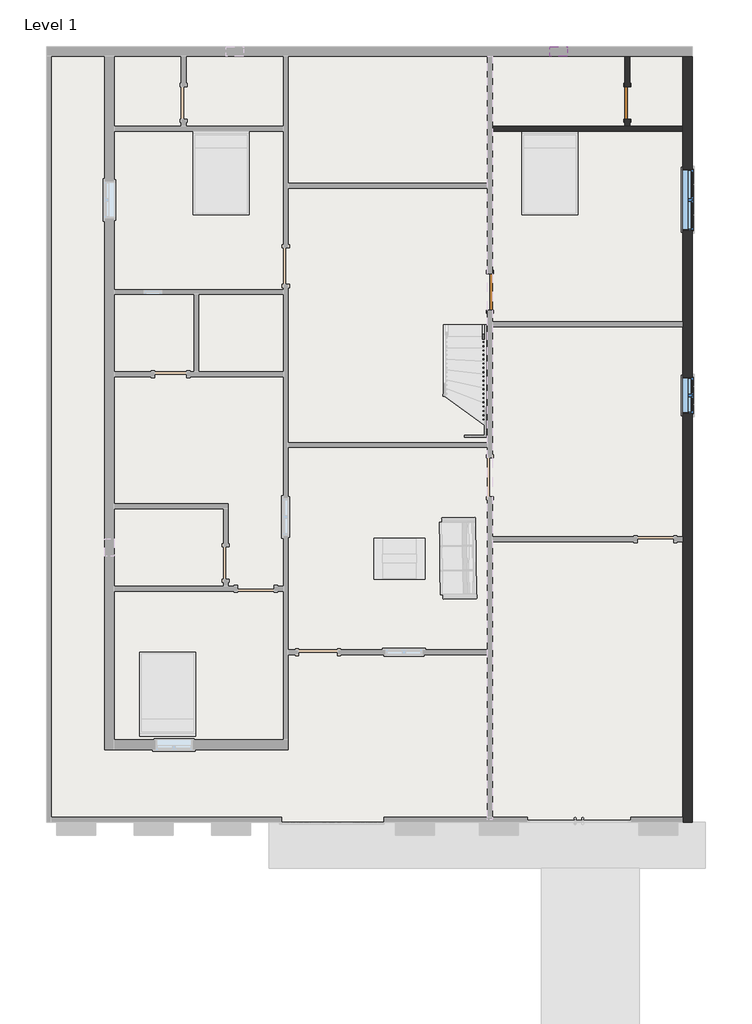
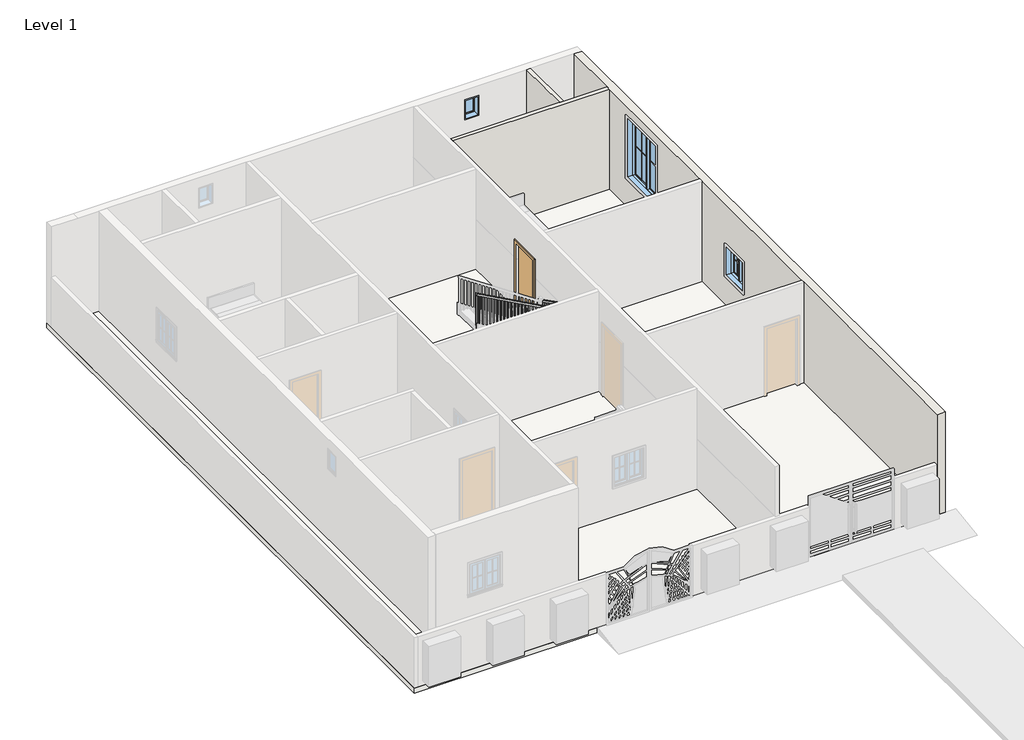
# One storey, part 2 of 3: 3 walls, 3 windows, 2 doors, 1 railing, 1 slab.
"""IFC4 building model written with IfcOpenShell, lengths in millimetres."""

from ifc_helpers import new_model, si_unit, frame, origin, place, context, project, spatial, polyline, outline, extrude, faceted_brep, transform, mapped, element, save
from components import door_f2b275c1, door_c29894e6, window_aa618e30, window_339605e1, window_9ac97e1a

model = new_model("IFC4")

# Units and contexts
model_context = context("Model", 3, world=origin())
ifc_project = project(units=[si_unit("LENGTHUNIT", "METRE", prefix="MILLI")], contexts=[model_context])

# Site, building, storey
site = spatial("IfcSite", under=ifc_project)
building = spatial("IfcBuilding", under=site)
storey = spatial("IfcBuildingStorey", under=building, Name="Level 1", Elevation=0.0)

# Doors
placement = place(None, origin())
door_shape = door_f2b275c1(model_context)
element("IfcDoor", 1, ObjectType="Single-Flush : 30\" x 80\"", at=placement, inside=storey, context=model_context, shape_type="MappedRepresentation", body=[
    mapped(door_shape, transform((4827.3366507, 9100.7522623, 0.0), x_axis=(0.0, -1.0, 0.0), y_axis=(1.0, 0.0, 0.0), z_axis=(0.0, 0.0, 1.0))),
])
door_2_shape = door_c29894e6(model_context)
element("IfcDoor", 2, ObjectType="Single-Flush : 34\" x 80\"", at=placement, inside=storey, context=model_context, shape_type="MappedRepresentation", body=[
    mapped(door_2_shape, transform((1583.2084916, 4643.0522623, 0.0), x_axis=(0.0, -1.0, 0.0), y_axis=(1.0, 0.0, 0.0), z_axis=(0.0, 0.0, 1.0))),
])

# Railing
element("IfcRailing", 3, ObjectType="Handrail - Rectangular", at=placement, inside=storey, context=model_context, shape_type="SolidModel", body=[
    faceted_brep([(1456.2084916, 3870.4222402, 1083.7333333), (1456.2084916, 3870.4222402, 1026.7391458), (1405.4084916, 3870.4222402, 1026.7391458), (1405.4084916, 3870.4222402, 1083.7333333), (1456.2084916, 1506.6647172, 2286.078212), (1456.2084916, 1494.487215, 2235.278212), (1405.4084916, 1494.487215, 2235.278212), (1405.4084916, 1506.6647172, 2286.078212), (1456.2084916, 1268.9652728, 2286.078212), (1456.2084916, 1268.9652728, 2235.278212), (1405.4084916, 1319.7652728, 2235.278212), (1405.4084916, 1319.7652728, 2286.078212), (1234.4478889, 1268.9652728, 2286.078212), (1221.4006723, 1268.9652728, 2235.278212), (1221.4006723, 1319.7652728, 2235.278212), (1234.4478889, 1319.7652728, 2286.078212), (-1813.7050583, 1268.9652728, 3962.4), (-1813.7050583, 1319.7652728, 3962.4), (-1813.7050583, 1319.7652728, 3904.4247257), (-1813.7050583, 1268.9652728, 3904.4247257)], [[[0, 1, 2, 3]], [[1, 0, 4, 5]], [[2, 1, 5, 6]], [[3, 2, 6, 7]], [[0, 3, 7, 4]], [[5, 4, 8, 9]], [[6, 5, 9, 10]], [[7, 6, 10, 11]], [[4, 7, 11, 8]], [[9, 8, 12, 13]], [[10, 9, 13, 14]], [[11, 10, 14, 15]], [[8, 11, 15, 12]], [[16, 17, 18, 19]], [[13, 12, 16, 19]], [[14, 13, 19, 18]], [[15, 14, 18, 17]], [[12, 15, 17, 16]]]),
    extrude(outline(polyline([(3857.4655707, -1728.3165084), (2878.6666667, -1728.3165084), (2878.6666667, -1709.2665084), (3846.9890853, -1709.2665084), (3857.4655707, -1728.3165084)])), frame((0.0, 1284.8402728, 0.0), z_axis=(0.0, 1.0, 0.0), x_axis=(0.0, 0.0, 1.0)), (0.0, 0.0, 1.0), 19.05),
    extrude(outline(polyline([(3801.5909816, -1626.7165084), (2878.6666667, -1626.7165084), (2878.6666667, -1607.6665084), (3791.1144961, -1607.6665084), (3801.5909816, -1626.7165084)])), frame((0.0, 1284.8402728, 0.0), z_axis=(0.0, 1.0, 0.0), x_axis=(0.0, 0.0, 1.0)), (0.0, 0.0, 1.0), 19.05),
    extrude(outline(polyline([(3745.7163924, -1525.1165084), (2709.3333333, -1525.1165084), (2709.3333333, -1506.0665084), (3735.2399069, -1506.0665084), (3745.7163924, -1525.1165084)])), frame((0.0, 1284.8402728, 0.0), z_axis=(0.0, 1.0, 0.0), x_axis=(0.0, 0.0, 1.0)), (0.0, 0.0, 1.0), 19.05),
    extrude(outline(polyline([(3689.8418032, -1423.5165084), (2709.3333333, -1423.5165084), (2709.3333333, -1404.4665084), (3679.3653177, -1404.4665084), (3689.8418032, -1423.5165084)])), frame((0.0, 1284.8402728, 0.0), z_axis=(0.0, 1.0, 0.0), x_axis=(0.0, 0.0, 1.0)), (0.0, 0.0, 1.0), 19.05),
    extrude(outline(polyline([(3633.967214, -1321.9165084), (2709.3333333, -1321.9165084), (2709.3333333, -1302.8665084), (3623.4907286, -1302.8665084), (3633.967214, -1321.9165084)])), frame((0.0, 1284.8402728, 0.0), z_axis=(0.0, 1.0, 0.0), x_axis=(0.0, 0.0, 1.0)), (0.0, 0.0, 1.0), 19.05),
    extrude(outline(polyline([(3578.0926249, -1220.3165084), (2540.0, -1220.3165084), (2540.0, -1201.2665084), (3567.6161394, -1201.2665084), (3578.0926249, -1220.3165084)])), frame((0.0, 1284.8402728, 0.0), z_axis=(0.0, 1.0, 0.0), x_axis=(0.0, 0.0, 1.0)), (0.0, 0.0, 1.0), 19.05),
    extrude(outline(polyline([(3522.2180357, -1118.7165084), (2540.0, -1118.7165084), (2540.0, -1099.6665084), (3511.7415502, -1099.6665084), (3522.2180357, -1118.7165084)])), frame((0.0, 1284.8402728, 0.0), z_axis=(0.0, 1.0, 0.0), x_axis=(0.0, 0.0, 1.0)), (0.0, 0.0, 1.0), 19.05),
    extrude(outline(polyline([(3466.3434465, -1017.1165084), (2540.0, -1017.1165084), (2540.0, -998.0665084), (3455.866961, -998.0665084), (3466.3434465, -1017.1165084)])), frame((0.0, 1284.8402728, 0.0), z_axis=(0.0, 1.0, 0.0), x_axis=(0.0, 0.0, 1.0)), (0.0, 0.0, 1.0), 19.05),
    extrude(outline(polyline([(3410.4688573, -915.5165084), (2370.6666667, -915.5165084), (2370.6666667, -896.4665084), (3399.9923719, -896.4665084), (3410.4688573, -915.5165084)])), frame((0.0, 1284.8402728, 0.0), z_axis=(0.0, 1.0, 0.0), x_axis=(0.0, 0.0, 1.0)), (0.0, 0.0, 1.0), 19.05),
    extrude(outline(polyline([(3354.5942682, -813.9165084), (2370.6666667, -813.9165084), (2370.6666667, -794.8665084), (3344.1177827, -794.8665084), (3354.5942682, -813.9165084)])), frame((0.0, 1284.8402728, 0.0), z_axis=(0.0, 1.0, 0.0), x_axis=(0.0, 0.0, 1.0)), (0.0, 0.0, 1.0), 19.05),
    extrude(outline(polyline([(3298.719679, -712.3165084), (2370.6666667, -712.3165084), (2370.6666667, -693.2665084), (3288.2431935, -693.2665084), (3298.719679, -712.3165084)])), frame((0.0, 1284.8402728, 0.0), z_axis=(0.0, 1.0, 0.0), x_axis=(0.0, 0.0, 1.0)), (0.0, 0.0, 1.0), 19.05),
    extrude(outline(polyline([(3242.8450898, -610.7165084), (2201.3333333, -610.7165084), (2201.3333333, -591.6665084), (3232.3686044, -591.6665084), (3242.8450898, -610.7165084)])), frame((0.0, 1284.8402728, 0.0), z_axis=(0.0, 1.0, 0.0), x_axis=(0.0, 0.0, 1.0)), (0.0, 0.0, 1.0), 19.05),
    extrude(outline(polyline([(3186.9705007, -509.1165084), (2201.3333333, -509.1165084), (2201.3333333, -490.0665084), (3176.4940152, -490.0665084), (3186.9705007, -509.1165084)])), frame((0.0, 1284.8402728, 0.0), z_axis=(0.0, 1.0, 0.0), x_axis=(0.0, 0.0, 1.0)), (0.0, 0.0, 1.0), 19.05),
    extrude(outline(polyline([(3131.0959115, -407.5165084), (2201.3333333, -407.5165084), (2201.3333333, -388.4665084), (3120.619426, -388.4665084), (3131.0959115, -407.5165084)])), frame((0.0, 1284.8402728, 0.0), z_axis=(0.0, 1.0, 0.0), x_axis=(0.0, 0.0, 1.0)), (0.0, 0.0, 1.0), 19.05),
    extrude(outline(polyline([(3075.2213223, -305.9165084), (2032.0, -305.9165084), (2032.0, -286.8665084), (3064.7448368, -286.8665084), (3075.2213223, -305.9165084)])), frame((0.0, 1284.8402728, 0.0), z_axis=(0.0, 1.0, 0.0), x_axis=(0.0, 0.0, 1.0)), (0.0, 0.0, 1.0), 19.05),
    extrude(outline(polyline([(3019.3467331, -204.3165084), (2032.0, -204.3165084), (2032.0, -185.2665084), (3008.8702477, -185.2665084), (3019.3467331, -204.3165084)])), frame((0.0, 1284.8402728, 0.0), z_axis=(0.0, 1.0, 0.0), x_axis=(0.0, 0.0, 1.0)), (0.0, 0.0, 1.0), 19.05),
    extrude(outline(polyline([(2963.472144, -102.7165084), (2032.0, -102.7165084), (2032.0, -83.6665084), (2952.9956585, -83.6665084), (2963.472144, -102.7165084)])), frame((0.0, 1284.8402728, 0.0), z_axis=(0.0, 1.0, 0.0), x_axis=(0.0, 0.0, 1.0)), (0.0, 0.0, 1.0), 19.05),
    extrude(outline(polyline([(2907.5975548, -1.1165084), (1862.6666667, -1.1165084), (1862.6666667, 17.9334916), (2897.1210693, 17.9334916), (2907.5975548, -1.1165084)])), frame((0.0, 1284.8402728, 0.0), z_axis=(0.0, 1.0, 0.0), x_axis=(0.0, 0.0, 1.0)), (0.0, 0.0, 1.0), 19.05),
    extrude(outline(polyline([(2851.7229656, 100.4834916), (1862.6666667, 100.4834916), (1862.6666667, 119.5334916), (2841.2464801, 119.5334916), (2851.7229656, 100.4834916)])), frame((0.0, 1284.8402728, 0.0), z_axis=(0.0, 1.0, 0.0), x_axis=(0.0, 0.0, 1.0)), (0.0, 0.0, 1.0), 19.05),
    extrude(outline(polyline([(2795.8483764, 202.0834916), (1862.6666667, 202.0834916), (1862.6666667, 221.1334916), (2785.371891, 221.1334916), (2795.8483764, 202.0834916)])), frame((0.0, 1284.8402728, 0.0), z_axis=(0.0, 1.0, 0.0), x_axis=(0.0, 0.0, 1.0)), (0.0, 0.0, 1.0), 19.05),
    extrude(outline(polyline([(2739.9737873, 303.6834916), (1693.3333333, 303.6834916), (1693.3333333, 322.7334916), (2729.4973018, 322.7334916), (2739.9737873, 303.6834916)])), frame((0.0, 1284.8402728, 0.0), z_axis=(0.0, 1.0, 0.0), x_axis=(0.0, 0.0, 1.0)), (0.0, 0.0, 1.0), 19.05),
    extrude(outline(polyline([(2684.0991981, 405.2834916), (1693.3333333, 405.2834916), (1693.3333333, 424.3334916), (2673.6227126, 424.3334916), (2684.0991981, 405.2834916)])), frame((0.0, 1284.8402728, 0.0), z_axis=(0.0, 1.0, 0.0), x_axis=(0.0, 0.0, 1.0)), (0.0, 0.0, 1.0), 19.05),
    extrude(outline(polyline([(2628.2246089, 506.8834916), (1693.3333333, 506.8834916), (1693.3333333, 525.9334916), (2617.7481235, 525.9334916), (2628.2246089, 506.8834916)])), frame((0.0, 1284.8402728, 0.0), z_axis=(0.0, 1.0, 0.0), x_axis=(0.0, 0.0, 1.0)), (0.0, 0.0, 1.0), 19.05),
    extrude(outline(polyline([(2572.3500198, 608.4834916), (1524.0, 608.4834916), (1524.0, 627.5334916), (2561.8735343, 627.5334916), (2572.3500198, 608.4834916)])), frame((0.0, 1284.8402728, 0.0), z_axis=(0.0, 1.0, 0.0), x_axis=(0.0, 0.0, 1.0)), (0.0, 0.0, 1.0), 19.05),
    extrude(outline(polyline([(2516.4754306, 710.0834916), (1524.0, 710.0834916), (1524.0, 729.1334916), (2505.9989451, 729.1334916), (2516.4754306, 710.0834916)])), frame((0.0, 1284.8402728, 0.0), z_axis=(0.0, 1.0, 0.0), x_axis=(0.0, 0.0, 1.0)), (0.0, 0.0, 1.0), 19.05),
    extrude(outline(polyline([(2460.6008414, 811.6834916), (1524.0, 811.6834916), (1524.0, 830.7334916), (2450.1243559, 830.7334916), (2460.6008414, 811.6834916)])), frame((0.0, 1284.8402728, 0.0), z_axis=(0.0, 1.0, 0.0), x_axis=(0.0, 0.0, 1.0)), (0.0, 0.0, 1.0), 19.05),
    extrude(outline(polyline([(2404.7262522, 913.2834916), (1524.0, 913.2834916), (1524.0, 932.3334916), (2394.2497668, 932.3334916), (2404.7262522, 913.2834916)])), frame((0.0, 1284.8402728, 0.0), z_axis=(0.0, 1.0, 0.0), x_axis=(0.0, 0.0, 1.0)), (0.0, 0.0, 1.0), 19.05),
    extrude(outline(polyline([(2348.8516631, 1014.8834916), (1354.6666667, 1014.8834916), (1354.6666667, 1033.9334916), (2338.3751776, 1033.9334916), (2348.8516631, 1014.8834916)])), frame((0.0, 1284.8402728, 0.0), z_axis=(0.0, 1.0, 0.0), x_axis=(0.0, 0.0, 1.0)), (0.0, 0.0, 1.0), 19.05),
    extrude(outline(polyline([(2292.9770739, 1116.4834916), (1354.6666667, 1116.4834916), (1354.6666667, 1135.5334916), (2282.5005884, 1135.5334916), (2292.9770739, 1116.4834916)])), frame((0.0, 1284.8402728, 0.0), z_axis=(0.0, 1.0, 0.0), x_axis=(0.0, 0.0, 1.0)), (0.0, 0.0, 1.0), 19.05),
    extrude(outline(polyline([(2237.1024847, 1218.0834916), (1354.6666667, 1218.0834916), (1354.6666667, 1237.1334916), (2226.6259992, 1237.1334916), (2237.1024847, 1218.0834916)])), frame((0.0, 1284.8402728, 0.0), z_axis=(0.0, 1.0, 0.0), x_axis=(0.0, 0.0, 1.0)), (0.0, 0.0, 1.0), 19.05),
    extrude(outline(polyline([(1338.7334916, 1284.8402728), (1319.6834916, 1284.8402728), (1319.6834916, 1303.8902728), (1338.7334916, 1303.8902728), (1338.7334916, 1284.8402728)])), frame((0.0, 0.0, 1354.6666667), z_axis=(0.0, 0.0, 1.0), x_axis=(1.0, 0.0, 0.0)), (0.0, 0.0, 1.0), 880.6115453),
    extrude(outline(polyline([(1440.3334916, 1339.9472402), (1440.3334916, 1320.8972402), (1421.2834916, 1320.8972402), (1421.2834916, 1339.9472402), (1440.3334916, 1339.9472402)])), frame((0.0, 0.0, 1354.6666667), z_axis=(0.0, 0.0, 1.0), x_axis=(1.0, 0.0, 0.0)), (0.0, 0.0, 1.0), 880.6115453),
    extrude(outline(polyline([(1440.3334916, 1441.5472402), (1440.3334916, 1422.4972402), (1421.2834916, 1422.4972402), (1421.2834916, 1441.5472402), (1440.3334916, 1441.5472402)])), frame((0.0, 0.0, 1354.6666667), z_axis=(0.0, 0.0, 1.0), x_axis=(1.0, 0.0, 0.0)), (0.0, 0.0, 1.0), 880.6115453),
    extrude(outline(polyline([(1543.1472402, 2210.5268864), (1543.1472402, 1354.6666667), (1524.0972402, 1354.6666667), (1524.0972402, 2220.216827), (1543.1472402, 2210.5268864)])), frame((1421.2834916, 0.0, 0.0), z_axis=(1.0, 0.0, 0.0), x_axis=(0.0, 1.0, 0.0)), (0.0, 0.0, 1.0), 19.05),
    extrude(outline(polyline([(1644.7472402, 2158.8472033), (1644.7472402, 1185.3333333), (1625.6972402, 1185.3333333), (1625.6972402, 2168.5371439), (1644.7472402, 2158.8472033)])), frame((1421.2834916, 0.0, 0.0), z_axis=(1.0, 0.0, 0.0), x_axis=(0.0, 1.0, 0.0)), (0.0, 0.0, 1.0), 19.05),
    extrude(outline(polyline([(1746.3472402, 2107.1675203), (1746.3472402, 1185.3333333), (1727.2972402, 1185.3333333), (1727.2972402, 2116.8574608), (1746.3472402, 2107.1675203)])), frame((1421.2834916, 0.0, 0.0), z_axis=(1.0, 0.0, 0.0), x_axis=(0.0, 1.0, 0.0)), (0.0, 0.0, 1.0), 19.05),
    extrude(outline(polyline([(1847.9472402, 2055.4878372), (1847.9472402, 1185.3333333), (1828.8972402, 1185.3333333), (1828.8972402, 2065.1777778), (1847.9472402, 2055.4878372)])), frame((1421.2834916, 0.0, 0.0), z_axis=(1.0, 0.0, 0.0), x_axis=(0.0, 1.0, 0.0)), (0.0, 0.0, 1.0), 19.05),
    extrude(outline(polyline([(1949.5472402, 2003.8081541), (1949.5472402, 1185.3333333), (1930.4972402, 1185.3333333), (1930.4972402, 2013.4980947), (1949.5472402, 2003.8081541)])), frame((1421.2834916, 0.0, 0.0), z_axis=(1.0, 0.0, 0.0), x_axis=(0.0, 1.0, 0.0)), (0.0, 0.0, 1.0), 19.05),
    extrude(outline(polyline([(2051.1472402, 1952.128471), (2051.1472402, 1016.0), (2032.0972402, 1016.0), (2032.0972402, 1961.8184116), (2051.1472402, 1952.128471)])), frame((1421.2834916, 0.0, 0.0), z_axis=(1.0, 0.0, 0.0), x_axis=(0.0, 1.0, 0.0)), (0.0, 0.0, 1.0), 19.05),
    extrude(outline(polyline([(2152.7472402, 1900.4487879), (2152.7472402, 1016.0), (2133.6972402, 1016.0), (2133.6972402, 1910.1387285), (2152.7472402, 1900.4487879)])), frame((1421.2834916, 0.0, 0.0), z_axis=(1.0, 0.0, 0.0), x_axis=(0.0, 1.0, 0.0)), (0.0, 0.0, 1.0), 19.05),
    extrude(outline(polyline([(2254.3472402, 1848.7691048), (2254.3472402, 1016.0), (2235.2972402, 1016.0), (2235.2972402, 1858.4590454), (2254.3472402, 1848.7691048)])), frame((1421.2834916, 0.0, 0.0), z_axis=(1.0, 0.0, 0.0), x_axis=(0.0, 1.0, 0.0)), (0.0, 0.0, 1.0), 19.05),
    extrude(outline(polyline([(2355.9472402, 1797.0894218), (2355.9472402, 1016.0), (2336.8972402, 1016.0), (2336.8972402, 1806.7793623), (2355.9472402, 1797.0894218)])), frame((1421.2834916, 0.0, 0.0), z_axis=(1.0, 0.0, 0.0), x_axis=(0.0, 1.0, 0.0)), (0.0, 0.0, 1.0), 19.05),
    extrude(outline(polyline([(2457.5472402, 1745.4097387), (2457.5472402, 846.6666667), (2438.4972402, 846.6666667), (2438.4972402, 1755.0996793), (2457.5472402, 1745.4097387)])), frame((1421.2834916, 0.0, 0.0), z_axis=(1.0, 0.0, 0.0), x_axis=(0.0, 1.0, 0.0)), (0.0, 0.0, 1.0), 19.05),
    extrude(outline(polyline([(2559.1472402, 1693.7300556), (2559.1472402, 846.6666667), (2540.0972402, 846.6666667), (2540.0972402, 1703.4199962), (2559.1472402, 1693.7300556)])), frame((1421.2834916, 0.0, 0.0), z_axis=(1.0, 0.0, 0.0), x_axis=(0.0, 1.0, 0.0)), (0.0, 0.0, 1.0), 19.05),
    extrude(outline(polyline([(2660.7472402, 1642.0503725), (2660.7472402, 846.6666667), (2641.6972402, 846.6666667), (2641.6972402, 1651.7403131), (2660.7472402, 1642.0503725)])), frame((1421.2834916, 0.0, 0.0), z_axis=(1.0, 0.0, 0.0), x_axis=(0.0, 1.0, 0.0)), (0.0, 0.0, 1.0), 19.05),
    extrude(outline(polyline([(2762.3472402, 1590.3706894), (2762.3472402, 677.3333333), (2743.2972402, 677.3333333), (2743.2972402, 1600.06063), (2762.3472402, 1590.3706894)])), frame((1421.2834916, 0.0, 0.0), z_axis=(1.0, 0.0, 0.0), x_axis=(0.0, 1.0, 0.0)), (0.0, 0.0, 1.0), 19.05),
    extrude(outline(polyline([(2863.9472402, 1538.6910064), (2863.9472402, 677.3333333), (2844.8972402, 677.3333333), (2844.8972402, 1548.3809469), (2863.9472402, 1538.6910064)])), frame((1421.2834916, 0.0, 0.0), z_axis=(1.0, 0.0, 0.0), x_axis=(0.0, 1.0, 0.0)), (0.0, 0.0, 1.0), 19.05),
    extrude(outline(polyline([(2965.5472402, 1487.0113233), (2965.5472402, 677.3333333), (2946.4972402, 677.3333333), (2946.4972402, 1496.7012638), (2965.5472402, 1487.0113233)])), frame((1421.2834916, 0.0, 0.0), z_axis=(1.0, 0.0, 0.0), x_axis=(0.0, 1.0, 0.0)), (0.0, 0.0, 1.0), 19.05),
    extrude(outline(polyline([(3067.1472402, 1435.3316402), (3067.1472402, 508.0), (3048.0972402, 508.0), (3048.0972402, 1445.0215808), (3067.1472402, 1435.3316402)])), frame((1421.2834916, 0.0, 0.0), z_axis=(1.0, 0.0, 0.0), x_axis=(0.0, 1.0, 0.0)), (0.0, 0.0, 1.0), 19.05),
    extrude(outline(polyline([(3168.7472402, 1383.6519571), (3168.7472402, 508.0), (3149.6972402, 508.0), (3149.6972402, 1393.3418977), (3168.7472402, 1383.6519571)])), frame((1421.2834916, 0.0, 0.0), z_axis=(1.0, 0.0, 0.0), x_axis=(0.0, 1.0, 0.0)), (0.0, 0.0, 1.0), 19.05),
    extrude(outline(polyline([(3270.3472402, 1331.972274), (3270.3472402, 508.0), (3251.2972402, 508.0), (3251.2972402, 1341.6622146), (3270.3472402, 1331.972274)])), frame((1421.2834916, 0.0, 0.0), z_axis=(1.0, 0.0, 0.0), x_axis=(0.0, 1.0, 0.0)), (0.0, 0.0, 1.0), 19.05),
    extrude(outline(polyline([(3371.9472402, 1280.2925909), (3371.9472402, 338.6666667), (3352.8972402, 338.6666667), (3352.8972402, 1289.9825315), (3371.9472402, 1280.2925909)])), frame((1421.2834916, 0.0, 0.0), z_axis=(1.0, 0.0, 0.0), x_axis=(0.0, 1.0, 0.0)), (0.0, 0.0, 1.0), 19.05),
    extrude(outline(polyline([(3473.5472402, 1228.6129079), (3473.5472402, 338.6666667), (3454.4972402, 338.6666667), (3454.4972402, 1238.3028484), (3473.5472402, 1228.6129079)])), frame((1421.2834916, 0.0, 0.0), z_axis=(1.0, 0.0, 0.0), x_axis=(0.0, 1.0, 0.0)), (0.0, 0.0, 1.0), 19.05),
    extrude(outline(polyline([(3575.1472402, 1176.9332248), (3575.1472402, 338.6666667), (3556.0972402, 338.6666667), (3556.0972402, 1186.6231654), (3575.1472402, 1176.9332248)])), frame((1421.2834916, 0.0, 0.0), z_axis=(1.0, 0.0, 0.0), x_axis=(0.0, 1.0, 0.0)), (0.0, 0.0, 1.0), 19.05),
    extrude(outline(polyline([(3676.7472402, 1125.2535417), (3676.7472402, 169.3333333), (3657.6972402, 169.3333333), (3657.6972402, 1134.9434823), (3676.7472402, 1125.2535417)])), frame((1421.2834916, 0.0, 0.0), z_axis=(1.0, 0.0, 0.0), x_axis=(0.0, 1.0, 0.0)), (0.0, 0.0, 1.0), 19.05),
    extrude(outline(polyline([(3778.3472402, 1073.5738586), (3778.3472402, 169.3333333), (3759.2972402, 169.3333333), (3759.2972402, 1083.2637992), (3778.3472402, 1073.5738586)])), frame((1421.2834916, 0.0, 0.0), z_axis=(1.0, 0.0, 0.0), x_axis=(0.0, 1.0, 0.0)), (0.0, 0.0, 1.0), 19.05),
    extrude(outline(polyline([(1440.3334916, 1303.8902728), (1440.3334916, 1284.8402728), (1421.2834916, 1284.8402728), (1421.2834916, 1303.8902728), (1440.3334916, 1303.8902728)])), frame((0.0, 0.0, 1354.6666667), z_axis=(0.0, 0.0, 1.0), x_axis=(1.0, 0.0, 0.0)), (0.0, 0.0, 1.0), 880.6115453),
    extrude(outline(polyline([(3904.4247257, -1813.7050583), (2878.6666667, -1813.7050583), (2878.6666667, -1794.6550583), (3893.9482402, -1794.6550583), (3904.4247257, -1813.7050583)])), frame((0.0, 1284.8402728, 0.0), z_axis=(0.0, 1.0, 0.0), x_axis=(0.0, 0.0, 1.0)), (0.0, 0.0, 1.0), 19.05),
    extrude(outline(polyline([(3870.4222402, 1026.7391458), (3870.4222402, 169.3333333), (3851.3722402, 169.3333333), (3851.3722402, 1036.4290864), (3870.4222402, 1026.7391458)])), frame((1421.2834916, 0.0, 0.0), z_axis=(1.0, 0.0, 0.0), x_axis=(0.0, 1.0, 0.0)), (0.0, 0.0, 1.0), 19.05),
])

# Slab
element("IfcSlab", 4, ObjectType="Generic - 12\"", at=placement, inside=storey, context=model_context, shape_type="SweptSolid", body=[
    extrude(outline(polyline([(6364.7584916, 10427.9022623), (6364.7584916, -7860.0977377), (-8875.2415084, -7860.0977377), (-8875.2415084, 10427.9022623), (6364.7584916, 10427.9022623)])), frame((0.0, 0.0, -152.4), z_axis=(0.0, 0.0, 1.0), x_axis=(1.0, 0.0, 0.0)), (0.0, 0.0, 1.0), 152.4),
])

# Walls
element("IfcWall", 5, ObjectType="9\"", at=placement, inside=storey, context=model_context, shape_type="Brep", body=[
    faceted_brep([(6136.1584916, 10199.3022623, 0.0), (6136.1584916, 8548.3022623, 0.0), (6136.1584916, 8434.0022623, 0.0), (6136.1584916, 3938.2022623, 0.0), (6136.1584916, 3823.9022623, 0.0), (6136.1584916, -1129.0977377, 0.0), (6136.1584916, -1243.3977377, 0.0), (6136.1584916, -7745.7977377, 0.0), (6136.1584916, -7860.0977377, 0.0), (6136.1584916, -7860.0977377, 1524.0), (6136.1584916, -7860.0977377, 3048.0), (6136.1584916, -1243.3977377, 3048.0), (6136.1584916, -1129.0977377, 3048.0), (6136.1584916, 3823.9022623, 3048.0), (6136.1584916, 3938.2022623, 3048.0), (6136.1584916, 8434.0022623, 3048.0), (6136.1584916, 8548.3022623, 3048.0), (6136.1584916, 10199.3022623, 3048.0), (6136.1584916, 1772.8522623, 1828.8), (6136.1584916, 1772.8522623, 914.4), (6136.1584916, 2636.4522623, 914.4), (6136.1584916, 2636.4522623, 1828.8), (6136.1584916, 6090.8522623, 2743.2), (6136.1584916, 6090.8522623, 914.4), (6136.1584916, 7538.6522623, 914.4), (6136.1584916, 7538.6522623, 2743.2), (6364.7584916, 10199.3022623, 0.0), (6364.7584916, 10199.3022623, 3048.0), (6364.7584916, -7860.0977377, 3048.0), (6364.7584916, -7860.0977377, 0.0), (6364.7584916, 1772.8522623, 1828.8), (6364.7584916, 2636.4522623, 1828.8), (6364.7584916, 2636.4522623, 914.4), (6364.7584916, 1772.8522623, 914.4), (6364.7584916, 6090.8522623, 2743.2), (6364.7584916, 7538.6522623, 2743.2), (6364.7584916, 7538.6522623, 914.4), (6364.7584916, 6090.8522623, 914.4)], [[[0, 1, 2, 3, 4, 5, 6, 7, 8, 9, 10, 11, 12, 13, 14, 15, 16, 17], [18, 19, 20, 21], [22, 23, 24, 25]], [[26, 27, 28, 29], [30, 31, 32, 33], [34, 35, 36, 37]], [[8, 7, 6, 5, 4, 3, 2, 1, 0, 26, 29]], [[0, 17, 27, 26]], [[10, 9, 8, 29, 28]], [[19, 18, 30, 33]], [[20, 19, 33, 32]], [[21, 20, 32, 31]], [[18, 21, 31, 30]], [[23, 22, 34, 37]], [[24, 23, 37, 36]], [[25, 24, 36, 35]], [[22, 25, 35, 34]], [[17, 16, 15, 14, 13, 12, 11, 10, 28, 27]]]),
])
element("IfcWall", 6, ObjectType="WALL4.5\"", at=placement, inside=storey, context=model_context, shape_type="SweptSolid", body=[
    extrude(outline(polyline([(8719.7522623, 2032.0), (8719.7522623, 0.0), (8548.3022623, 0.0), (8548.3022623, 3048.0), (10199.3022623, 3048.0), (10199.3022623, 0.0), (9481.7522623, 0.0), (9481.7522623, 2032.0), (8719.7522623, 2032.0)])), frame((4770.1866507, 0.0, 0.0), z_axis=(1.0, 0.0, 0.0), x_axis=(0.0, 1.0, 0.0)), (0.0, 0.0, 1.0), 114.3),
])
element("IfcWall", 7, ObjectType="WALL4.5\"", at=placement, inside=storey, context=model_context, shape_type="Brep", body=[
    faceted_brep([(1640.3584916, 8434.0022623, 0.0), (6136.1584916, 8434.0022623, 0.0), (6136.1584916, 8434.0022623, 3048.0), (1640.3584916, 8434.0022623, 3048.0), (1640.3584916, 8548.3022623, 0.0), (1640.3584916, 8548.3022623, 3048.0), (4770.1866507, 8548.3022623, 3048.0), (4884.4866507, 8548.3022623, 3048.0), (6136.1584916, 8548.3022623, 3048.0), (6136.1584916, 8548.3022623, 0.0), (4884.4866507, 8548.3022623, 0.0), (4770.1866507, 8548.3022623, 0.0)], [[[0, 1, 2, 3]], [[4, 5, 6, 7, 8, 9, 10, 11]], [[1, 0, 4, 11, 10, 9]], [[2, 1, 9, 8]], [[0, 3, 5, 4]], [[3, 2, 8, 7, 6, 5]]]),
])

# Windows
window_shape = window_aa618e30(model_context)
element("IfcWindow", 8, ObjectType="Fixed : 16\" x 24\"", at=placement, inside=storey, context=model_context, shape_type="MappedRepresentation", body=[
    mapped(window_shape, transform((3243.3725711, 10313.6022623, 1219.2), x_axis=(1.0, 0.0, 0.0), y_axis=(0.0, 1.0, 0.0), z_axis=(0.0, 0.0, 1.0))),
])
window_2_shape = window_339605e1(model_context)
element("IfcWindow", 9, ObjectType="Window-Casement-Double : 34\" x 36\"", at=placement, inside=storey, context=model_context, shape_type="MappedRepresentation", body=[
    mapped(window_2_shape, transform((6250.4584916, 2204.6522623, 0.0), x_axis=(0.0, -1.0, 0.0), y_axis=(1.0, 0.0, 0.0), z_axis=(0.0, 0.0, 1.0))),
])
window_3_shape = window_9ac97e1a(model_context)
element("IfcWindow", 10, ObjectType="Window-Casement-Double : 57\" x 72\"", at=placement, inside=storey, context=model_context, shape_type="MappedRepresentation", body=[
    mapped(window_3_shape, transform((6250.4584916, 6814.7522623, 0.0), x_axis=(0.0, -1.0, 0.0), y_axis=(1.0, 0.0, 0.0), z_axis=(0.0, 0.0, 1.0))),
])

save(model, "model.ifc")

# Revit data of these elements
# Type "Single-Flush : 30\" x 80\""
#   Type Mark = "5"
#   Construction Type Id = "MDOOR"
#   Assembly Code = "C1020"
#   Analytic Construction = "Metal"
#   Thickness = 0' - 2"
#   Heat Transfer Coefficient (U) = 0.651978 BTU/(h·ft²·°F)
#   Height = 6' - 8"
#   Trim Projection Ext = 0' - 1"
#   Trim Projection Int = 0' - 1"
#   Trim Width = 0' - 3"
#   Width = 2' - 6"
#   Define Thermal Properties by = 1
#   Define Thermal Properties by = 1
#   Door Material = Door - Panel
#   Frame Material = Door - Frame
#   Visual Light Transmittance = 0
#   Solar Heat Gain Coefficient = 0
#   Function = (empty or 0)
#   Wall Closure = (empty or 0)
# Type "Single-Flush : 34\" x 80\""
#   Type Mark = "7"
#   Construction Type Id = "MDOOR"
#   Assembly Code = "C1020"
#   Analytic Construction = "Metal"
#   Thickness = 0' - 2"
#   Heat Transfer Coefficient (U) = 0.651978 BTU/(h·ft²·°F)
#   Height = 6' - 8"
#   Trim Projection Ext = 0' - 1"
#   Trim Projection Int = 0' - 1"
#   Trim Width = 0' - 3"
#   Width = 2' - 10"
#   Define Thermal Properties by = 1
#   Define Thermal Properties by = 1
#   Door Material = Door - Panel
#   Frame Material = Door - Frame
#   Visual Light Transmittance = 0
#   Solar Heat Gain Coefficient = 0
#   Function = (empty or 0)
#   Wall Closure = (empty or 0)
# Type "Handrail - Rectangular"
#   Assembly Code = "C2010400"
#   built-in parameter 1008612 = 0.0416667 (stored number, unit not read)
#   built-in parameter 1008611 = 0.0416667 (stored number, unit not read)
#   built-in parameter 1008609 = 0.333333 (stored number, unit not read)
#   built-in parameter 1008604 = 0.166667 (stored number, unit not read)
#   built-in parameter 1008603 = 0.166667 (stored number, unit not read)
#   Railing Height = 3' - 0"
#   built-in parameter 1008630 = 2
#   built-in parameter 1008610 = 2
#   built-in parameter 1008618 = Baluster - Square : 3/4"
# Type "Generic - 12\""
#   Assembly Code = "B1010"
#   Function = 0
#   Layers, outside or top first: 0' - 6" no material (function 1)
# Type "9\""
#   Assembly Code = "B2010"
#   Layers, outside or top first: 0' - 9" no material (function 1)
# Type "WALL4.5\""
#   Assembly Code = "B2010"
#   Layers, outside or top first: 0' - 4 1/2" no material (function 1)
# Type "Fixed : 16\" x 24\""
#   Type Mark = "4"
#   Construction Type Id = "GSP4R"
#   Assembly Code = "B2020100"
#   Analytic Construction = "1/8 in Pilkington single glazing"
#   Visual Light Transmittance = 0.9
#   Solar Heat Gain Coefficient = 0.78
#   Heat Transfer Coefficient (U) = 0.6496 BTU/(h·ft²·°F)
#   Height = 2' - 0"
#   Default Sill Height = 3' - 0"
#   Width = 1' - 4"
#   Window Inset = 0' - 0 3/4"
#   Define Thermal Properties by = 1
#   Define Thermal Properties by = 1
#   Glass Pane Material = Glass
#   Sash Material = Sash
#   Wall Closure = (empty or 0)
# Type "Window-Casement-Double : 34\" x 36\""
#   Type Mark = "14"
#   Fire Rating = "0.5h"
#   Assembly Code = "B2020100"
#   Analytic Construction = "Double glazing - domestic"
#   Frame Extension [instance default] = 0' - 0 1/4"
#   Window Inset [instance default] = 0' - 0"
#   Wall Thickness [instance default] = 0' - 6"
#   Interior Wall Closure [instance default] = 0' - 2 1/4"
#   Half Width = 1' - 5"
#   Visual Light Transmittance = 0.81
#   Thermal Resistance (R) = 1.8146 (h·ft²·°F)/BTU
#   Solar Heat Gain Coefficient = 0.76
#   Rough Width = 2' - 10 1/2"
#   Rough Height = 3' - 0 1/2"
#   Height = 3' - 0"
#   Heat Transfer Coefficient (U) = 0.5511 BTU/(h·ft²·°F)
#   Exterior Wall Closure [instance default] = 0' - 1 1/4"
#   Extension Jamb [instance default] = 0' - 2 1/4"
#   Default Sill Height = 3' - 0"
#   Width = 2' - 10"
#   Define Thermal Properties by = 0
#   Muntin Visibility = yes
#   Interior Trim Visibility [instance default] = yes
#   Exterior Trim Visibility [instance default] = yes
#   Extension Jamb Visibility [instance default] = yes
#   Interior Trim Material = Wood - Stained
#   Muntin Pattern = Muntin Pattern_2x2 : Muntin Pattern_2x2
#   Interior Trim = Trim-Window-Interior-Flat : Picture Frame
#   Interior Frame Material = Wood - Stained
#   Glass Panel Material = Glass
#   Exterior Trim Material = Clad - White
#   Exterior Trim = Trim-Window-Exterior-Flat : with Sill
#   Exterior Frame Material = Clad - White
#   Wall Closure = (empty or 0)
# Type "Window-Casement-Double : 57\" x 72\""
#   Type Mark = "17"
#   Fire Rating = "0.5h"
#   Assembly Code = "B2020100"
#   Analytic Construction = "Double glazing - domestic"
#   Frame Extension [instance default] = 0' - 0 1/4"
#   Window Inset [instance default] = 0' - 0"
#   Wall Thickness [instance default] = 0' - 6"
#   Interior Wall Closure [instance default] = 0' - 2 1/4"
#   Half Width = 2' - 4 1/2"
#   Visual Light Transmittance = 0.81
#   Thermal Resistance (R) = 1.8146 (h·ft²·°F)/BTU
#   Solar Heat Gain Coefficient = 0.76
#   Rough Width = 4' - 9 1/2"
#   Rough Height = 6' - 0 1/2"
#   Height = 6' - 0"
#   Heat Transfer Coefficient (U) = 0.5511 BTU/(h·ft²·°F)
#   Exterior Wall Closure [instance default] = 0' - 1 1/4"
#   Extension Jamb [instance default] = 0' - 2 1/4"
#   Default Sill Height = 3' - 0"
#   Width = 4' - 9"
#   Define Thermal Properties by = 0
#   Muntin Visibility = yes
#   Interior Trim Visibility [instance default] = yes
#   Exterior Trim Visibility [instance default] = yes
#   Extension Jamb Visibility [instance default] = yes
#   Interior Trim Material = Wood - Stained
#   Muntin Pattern = Muntin Pattern_2x2 : Muntin Pattern_2x2
#   Interior Trim = Trim-Window-Interior-Flat : Picture Frame
#   Interior Frame Material = Wood - Stained
#   Glass Panel Material = Glass
#   Exterior Trim Material = Clad - White
#   Exterior Trim = Trim-Window-Exterior-Flat : with Sill
#   Exterior Frame Material = Clad - White
#   Wall Closure = (empty or 0)
# Element 1 (IfcDoor, "Single-Flush : 30\" x 80\"")
#   Phase Created = New Construction
#   Materials on its faces: "Door - Frame", "Door - Panel"
# Element 2 (IfcDoor, "Single-Flush : 34\" x 80\"")
#   Phase Created = New Construction
#   Materials on its faces: "Door - Frame", "Door - Panel"
# Element 3 (IfcRailing, "Handrail - Rectangular")
#   Phase Created = New Construction
# Element 4 (IfcSlab, "Generic - 12\"")
#   Height Offset From Level = 0' - 0"
#   Phase Created = New Construction
#   Materials on its faces: "Default Floor"
# Element 5 (IfcWall, "9\"")
#   Top Offset = 0' - 0"
#   Base Offset = 0' - 0"
#   Unconnected Height = 10' - 0"
#   wall height = 10' - 0"
#   Phase Created = New Construction
#   Base Constraint = Level 1
#   Materials on its faces: "Default Wall", "legs"
# Elements 6, 7 (IfcWall, "WALL4.5\"")
#   Top Offset = 0' - 0"
#   Base Offset = 0' - 0"
#   Unconnected Height = 10' - 0"
#   wall height = 10' - 0"
#   Phase Created = New Construction
#   Base Constraint = Level 1
#   Materials on its faces: "Default Wall"
# Element 8 (IfcWindow, "Fixed : 16\" x 24\"")
#   Mark = "2"
#   Phase Created = New Construction
#   Materials on its faces: "Sash", "Glass"
# Element 9 (IfcWindow, "Window-Casement-Double : 34\" x 36\"")
#   Mark = "8"
#   Window Inset = 0' - 0"
#   Interior Wall Closure = 0' - 2 1/4"
#   Frame Extension = 0' - 0 1/4"
#   Exterior Wall Closure = 0' - 1 1/4"
#   Interior Trim Visibility = yes
#   Exterior Trim Visibility = yes
#   Phase Created = New Construction
#   Materials on its faces: "Wood - Stained", "Glass", "Clad - White"
# Element 10 (IfcWindow, "Window-Casement-Double : 57\" x 72\"")
#   Mark = "9"
#   Window Inset = 0' - 0"
#   Interior Wall Closure = 0' - 2 1/4"
#   Frame Extension = 0' - 0 1/4"
#   Exterior Wall Closure = 0' - 1 1/4"
#   Interior Trim Visibility = yes
#   Exterior Trim Visibility = yes
#   Phase Created = New Construction
#   Materials on its faces: "Wood - Stained", "Glass", "Clad - White"
# Materials
#   "Door - Panel": class "Wood", colour RGB 210 159 95, transparency 0, Cost = 0
#   "Door - Frame": colour RGB 118 70 51, transparency 0, Cost = 0
#   "Glass": class "Glass", colour RGB 0 128 192, transparency 0.75, Description = "Soda Lime Glass", Cost = 0
#   "Sash": class "Wood", colour RGB 224 178 126, transparency 0, Cost = 0
#   "Wood - Stained": class "Wood", colour RGB 224 178 126, transparency 0, Cost = 0
#   "Clad - White": class "Wood", colour RGB 242 242 238, transparency 0, Cost = 0
#   "Default Floor": colour RGB 128 128 128, transparency 0, Cost = 0
#   "Default Wall": colour RGB 128 128 128, transparency 0, Cost = 0
#   "legs": colour RGB 90 73 37, transparency 0, Cost = 0
